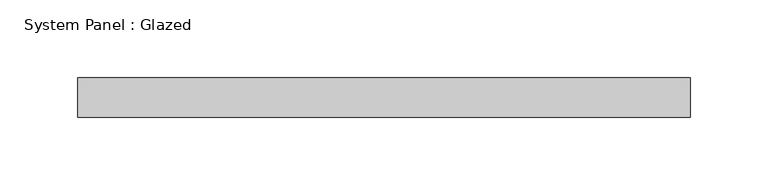
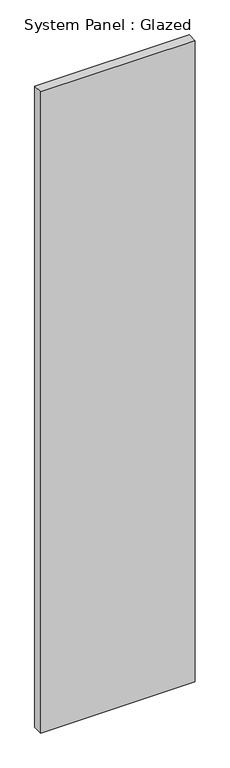
"""IFC4 building model written with IfcOpenShell, lengths in millimetres: plate geometry, System Panel : Glazed."""

from ifc_helpers import new_model, si_unit, origin, origin_with_axes, place, context, project, spatial, polyline, outline, extrude, source, transform, mapped, element, save


def system_panel_glazed_27f64093(model_context):
    return source(origin(), model_context, "Body", "SweptSolid", [
        extrude(outline(polyline([(196.85, 19.05), (-196.85, 19.05), (-196.85, 44.45), (196.85, 44.45), (196.85, 19.05)])), origin_with_axes(), (0.0, 0.0, 1.0), 1725.7814546),
    ])


if __name__ == "__main__":
    model = new_model("IFC4")
    model_context = context("Model", 3, world=origin())
    ifc_project = project(units=[si_unit("LENGTHUNIT", "METRE", prefix="MILLI")], contexts=[model_context])
    site = spatial("IfcSite", under=ifc_project)
    building = spatial("IfcBuilding", under=site)
    placement = place(None, origin())
    system_panel_glazed_shape = system_panel_glazed_27f64093(model_context)
    element("IfcPlate", 1, ObjectType="System Panel : Glazed", at=placement, inside=building, context=model_context, shape_type="MappedRepresentation", body=[
        mapped(system_panel_glazed_shape, transform((0.0, 0.0, 0.0), x_axis=(1.0, 0.0, 0.0), y_axis=(0.0, 1.0, 0.0), z_axis=(0.0, 0.0, 1.0))),
    ])
    save(model, "model.ifc")

# Revit data of these elements
# Type "System Panel : Glazed"
#   Construction Type Id = "GSP4R"
#   Analytic Construction = "1/8 in Pilkington single glazing"
#   Visual Light Transmittance = 0.9
#   Solar Heat Gain Coefficient = 0.86
#   Heat Transfer Coefficient (U) = 1.18115 BTU/(h·ft²·°F)
#   Define Thermal Properties by = 1
# Element 1 (IfcPlate, "System Panel : Glazed")
#   Materials on its faces: "Glass"
# Materials
#   "Glass": class "Glass", colour RGB 0 128 192, transparency 0.75, Description = "Soda Lime Glass", Cost = 0
